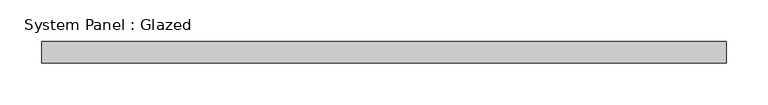
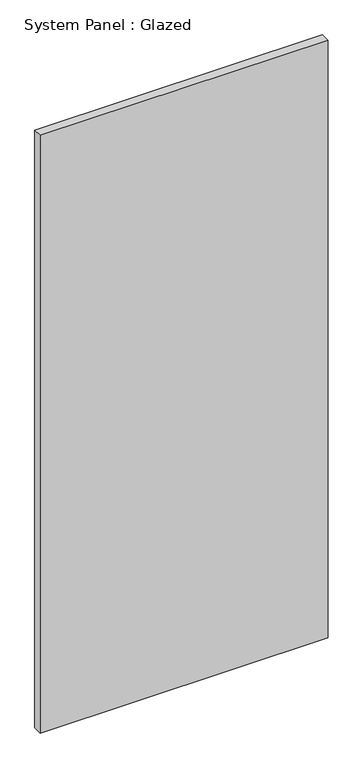
"""IFC4 building model written with IfcOpenShell, lengths in millimetres: plate geometry, System Panel : Glazed."""

from ifc_helpers import new_model, si_unit, origin, origin_with_axes, place, context, project, spatial, polyline, outline, extrude, source, transform, mapped, element, save


def system_panel_glazed_6230de04(model_context):
    return source(origin(), model_context, "Body", "SweptSolid", [
        extrude(outline(polyline([(409.575, 19.05), (-409.575, 19.05), (-409.575, 44.45), (409.575, 44.45), (409.575, 19.05)])), origin_with_axes(), (0.0, 0.0, 1.0), 1797.05),
    ])


if __name__ == "__main__":
    model = new_model("IFC4")
    model_context = context("Model", 3, world=origin())
    ifc_project = project(units=[si_unit("LENGTHUNIT", "METRE", prefix="MILLI")], contexts=[model_context])
    site = spatial("IfcSite", under=ifc_project)
    building = spatial("IfcBuilding", under=site)
    placement = place(None, origin())
    system_panel_glazed_shape = system_panel_glazed_6230de04(model_context)
    element("IfcPlate", 1, ObjectType="System Panel : Glazed", at=placement, inside=building, context=model_context, shape_type="MappedRepresentation", body=[
        mapped(system_panel_glazed_shape, transform((0.0, 0.0, 0.0), x_axis=(1.0, 0.0, 0.0), y_axis=(0.0, 1.0, 0.0), z_axis=(0.0, 0.0, 1.0))),
    ])
    save(model, "model.ifc")

# Revit data of these elements
# Type "System Panel : Glazed"
#   Construction Type Id = "GSP4R"
#   Analytic Construction = "1/8 in Pilkington single glazing"
#   Visual Light Transmittance = 0.9
#   Solar Heat Gain Coefficient = 0.86
#   Heat Transfer Coefficient (U) = 6.7069 W/(m²·K)
# Element 1 (IfcPlate, "System Panel : Glazed")
#   Materials on its faces: "Glass"
# Materials
#   "Glass": class "Glass", colour RGB 0 128 192, transparency 0.75, Description = "Soda Lime Glass", Cost = 0
